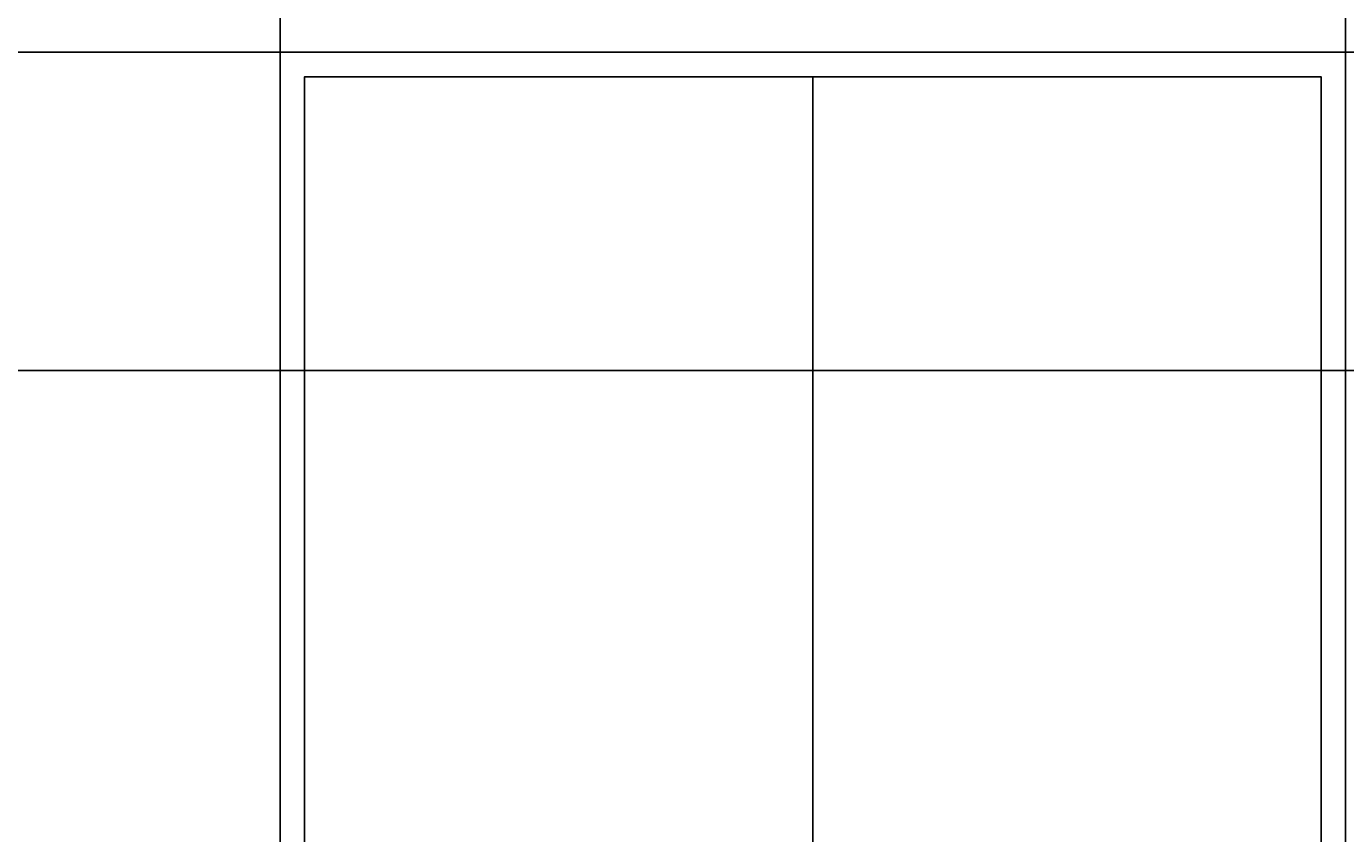
# Model space of a CAD drawing. Units: inches. Extents: x -145 to 510, y 5 to 386.
# Tile 12 of 25: x 75 to 182, y 242 to 308. Entities that reach past the tile are written whole.
import ezdxf

# ---------------------------------------------------------------- set-up
doc = ezdxf.new("R2010")
doc.units = ezdxf.units.IN
doc.header["$MEASUREMENT"] = 0
doc.layers.add('A-ANNO-DIMS', color=2, linetype='Continuous', lineweight=18)
doc.layers.add('A-GLAZ', color=4, linetype='Continuous', lineweight=25)
doc.styles.get("Standard").update_dxf_attribs({"font": 'arial.ttf'})
doc.dimstyles.get("Standard").update_dxf_attribs({"dimtxt": 0.6875, "dimasz": 0.18, "dimexe": 0.18, "dimexo": 0.0625, "dimgap": 0.09, "dimtad": 0, "dimtih": 1, "dimtoh": 1, "dimdec": 4, "dimzin": 0, "dimdsep": 46, "dimlunit": 4, "dimtxsty": 'Standard', "dimcen": 0.09, "dimadec": 0, "dimazin": 0, "dimtfac": 1, "dimtdec": 4, "dimtofl": 0, "dimtmove": 0, "dimatfit": 3, "dimfxl": 1, "dimtolj": 1, "dimtzin": 0, "dimarcsym": 0})

# ---------------------------------------------------------------- blocks, each defined once
blk = doc.blocks.new('*D15')
at = {"layer": 'A-ANNO-DIMS', "color": 0, "lineweight": -2, "transparency": 16777216}
for p, q in [((69.78, 199.95), (69.78, 385.97)), ((69.96, 385.79), (80.93, 385.79)), ((94.96, 385.79), (83.98, 385.79)), ((95.14, 305.8), (95.14, 385.97))]:
    blk.add_line(p, q, dxfattribs=at)
at = {"layer": 'A-ANNO-DIMS', "color": 0, "transparency": 16777216}
for points in [[(69.96, 385.82), (69.96, 385.76), (69.78, 385.79)], [(94.96, 385.82), (94.96, 385.76), (95.14, 385.79)]]:
    blk.add_solid(points, dxfattribs=at)
at = {"layer": 'Defpoints', "color": 0, "transparency": 16777216}
for p in [(95.14, 385.79), (95.14, 305.74), (69.78, 199.89)]:
    blk.add_point(p, dxfattribs=at)
at = {"layer": 'A-ANNO-DIMS', "color": 0, "transparency": 16777216, "insert": (82.46, 385.79), "char_height": 0.688, "attachment_point": 5}
blk.add_mtext('\\A1;25.365', dxfattribs=at)
blk = doc.blocks.new('*D16')
at = {"layer": 'A-ANNO-DIMS', "color": 0, "lineweight": -2, "transparency": 16777216}
for p, q in [((95.14, 305.8), (95.14, 385.97)), ((95.32, 385.79), (137.23, 385.79)), ((181.64, 385.79), (139.73, 385.79)), ((181.82, 305.8), (181.82, 385.97))]:
    blk.add_line(p, q, dxfattribs=at)
at = {"layer": 'A-ANNO-DIMS', "color": 0, "transparency": 16777216}
for points in [[(95.32, 385.82), (95.32, 385.76), (95.14, 385.79)], [(181.64, 385.82), (181.64, 385.76), (181.82, 385.79)]]:
    blk.add_solid(points, dxfattribs=at)
at = {"layer": 'Defpoints', "color": 0, "transparency": 16777216}
for p in [(181.82, 385.79), (95.14, 305.74), (181.82, 305.74)]:
    blk.add_point(p, dxfattribs=at)
at = {"layer": 'A-ANNO-DIMS', "color": 0, "transparency": 16777216, "insert": (138.48, 385.79), "char_height": 0.688, "attachment_point": 5}
blk.add_mtext('\\A1;86.68', dxfattribs=at)
blk = doc.blocks.new('*D19')
at = {"layer": 'A-ANNO-DIMS', "color": 0, "lineweight": -2, "transparency": 16777216}
for p, q in [((478.76, 355.89), (-144.05, 355.89)), ((-143.87, 355.71), (-143.87, 218.33)), ((-143.87, 80.07), (-143.87, 217.45)), ((-114.04, 79.89), (-144.05, 79.89))]:
    blk.add_line(p, q, dxfattribs=at)
at = {"layer": 'A-ANNO-DIMS', "color": 0, "transparency": 16777216}
for points in [[(-143.9, 355.71), (-143.84, 355.71), (-143.87, 355.89)], [(-143.9, 80.07), (-143.84, 80.07), (-143.87, 79.89)]]:
    blk.add_solid(points, dxfattribs=at)
at = {"layer": 'Defpoints', "color": 0, "transparency": 16777216}
for p in [(-143.87, 355.89), (478.83, 355.89), (-113.97, 79.89)]:
    blk.add_point(p, dxfattribs=at)
at = {"layer": 'A-ANNO-DIMS', "color": 0, "transparency": 16777216, "insert": (-143.87, 217.89), "char_height": 0.688, "attachment_point": 5}
blk.add_mtext('\\A1;276', dxfattribs=at)
blk = doc.blocks.new('*D26')
at = {"layer": 'A-ANNO-DIMS', "color": 0, "lineweight": -2, "transparency": 16777216}
for p, q in [((95.08, 305.74), (-144.05, 305.74)), ((-143.87, 305.56), (-143.87, 253.26)), ((-143.87, 200.07), (-143.87, 252.38)), ((95.08, 199.89), (-144.05, 199.89))]:
    blk.add_line(p, q, dxfattribs=at)
at = {"layer": 'A-ANNO-DIMS', "color": 0, "transparency": 16777216}
for points in [[(-143.9, 305.56), (-143.84, 305.56), (-143.87, 305.74)], [(-143.9, 200.07), (-143.84, 200.07), (-143.87, 199.89)]]:
    blk.add_solid(points, dxfattribs=at)
at = {"layer": 'Defpoints', "color": 0, "transparency": 16777216}
for p in [(-143.87, 305.74), (95.14, 305.74), (95.14, 199.89)]:
    blk.add_point(p, dxfattribs=at)
at = {"layer": 'A-ANNO-DIMS', "color": 0, "transparency": 16777216, "insert": (-143.87, 252.82), "char_height": 0.688, "attachment_point": 5}
blk.add_mtext('\\A1;105.85', dxfattribs=at)
blk = doc.blocks.new('*D27')
at = {"layer": 'A-ANNO-DIMS', "color": 0, "lineweight": -2, "transparency": 16777216}
for p, q in [((244.23, 279.84), (-144.05, 279.84)), ((-143.87, 279.66), (-143.87, 240.31)), ((-143.87, 200.07), (-143.87, 239.43)), ((218.29, 199.89), (-144.05, 199.89))]:
    blk.add_line(p, q, dxfattribs=at)
at = {"layer": 'A-ANNO-DIMS', "color": 0, "transparency": 16777216}
for points in [[(-143.9, 279.66), (-143.84, 279.66), (-143.87, 279.84)], [(-143.9, 200.07), (-143.84, 200.07), (-143.87, 199.89)]]:
    blk.add_solid(points, dxfattribs=at)
at = {"layer": 'Defpoints', "color": 0, "transparency": 16777216}
for p in [(-143.87, 279.84), (244.29, 279.84), (218.36, 199.89)]:
    blk.add_point(p, dxfattribs=at)
at = {"layer": 'A-ANNO-DIMS', "color": 0, "transparency": 16777216, "insert": (-143.87, 239.87), "char_height": 0.688, "attachment_point": 5}
blk.add_mtext('\\A1;79.95', dxfattribs=at)
blk = doc.blocks.new('*D28')
at = {"layer": 'A-ANNO-DIMS', "color": 0, "lineweight": -2, "transparency": 16777216}
for p, q in [((244.23, 305.74), (-144.05, 305.74)), ((-143.87, 305.56), (-143.87, 293.23)), ((-143.87, 280.02), (-143.87, 292.35)), ((244.23, 279.84), (-144.05, 279.84))]:
    blk.add_line(p, q, dxfattribs=at)
at = {"layer": 'A-ANNO-DIMS', "color": 0, "transparency": 16777216}
for points in [[(-143.9, 305.56), (-143.84, 305.56), (-143.87, 305.74)], [(-143.9, 280.02), (-143.84, 280.02), (-143.87, 279.84)]]:
    blk.add_solid(points, dxfattribs=at)
at = {"layer": 'Defpoints', "color": 0, "transparency": 16777216}
for p in [(-143.87, 305.74), (244.29, 305.74), (244.29, 279.84)]:
    blk.add_point(p, dxfattribs=at)
at = {"layer": 'A-ANNO-DIMS', "color": 0, "transparency": 16777216, "insert": (-143.87, 292.79), "char_height": 0.688, "attachment_point": 5}
blk.add_mtext('\\A1;25.897', dxfattribs=at)

msp = doc.modelspace()

# ---------------------------------------------------------------- linework, layer by layer
at = {"layer": 'A-GLAZ'}
msp.add_line((138.4805, 303.7416), (138.4805, 201.8905), dxfattribs=at)
for points in [[(95.1414, 199.8905), (181.8195, 199.8905), (181.8195, 305.7416), (95.1414, 305.7416)], [(97.1414, 201.8905), (179.8195, 201.8905), (179.8195, 303.7416), (97.1414, 303.7416)]]:
    msp.add_lwpolyline(points, close=True, dxfattribs=at)

# ---------------------------------------------------------------- dimensions: what is measured, and where the dimension line sits
at = {"layer": 'A-ANNO-DIMS'}
for base, p1, p2, override, picture, middle in [((95.1414, 385.7905), (69.7763, 199.8905), (95.1414, 305.7416), {"dimdec": 3, "dimlfac": 1, "dimrnd": 0, "dimzin": 0, "dimdsep": 46, "dimlunit": 2}, '*D15', (82.4589, 385.7905)), ((181.8195, 385.7905), (95.1414, 305.7416), (181.8195, 305.7416), {"dimdec": 2, "dimlfac": 1, "dimrnd": 0, "dimzin": 0, "dimdsep": 46, "dimlunit": 2}, '*D16', (138.4805, 385.7905))]:
    dim = msp.add_linear_dim(base=base, p1=p1, p2=p2, dimstyle='Standard', override=override, dxfattribs=at)
    dim.commit()
    dim.dimension.update_dxf_attribs({"geometry": picture, "text_midpoint": middle})
for base, p1, p2, override, picture, middle in [((-143.8737, 355.8905), (-113.9737, 79.8905), (478.8263, 355.8905), {"dimdec": 0, "dimlfac": 1, "dimrnd": 0, "dimzin": 0, "dimdsep": 46, "dimlunit": 2}, '*D19', (-143.8737, 217.8905)), ((-143.8737, 305.7416), (95.1414, 199.8905), (95.1414, 305.7416), {"dimdec": 2, "dimlfac": 1, "dimrnd": 0, "dimzin": 0, "dimdsep": 46, "dimlunit": 2}, '*D26', (-143.8737, 252.8161)), ((-143.8737, 305.7416), (244.2916, 279.8443), (244.2916, 305.7416), {"dimdec": 3, "dimlfac": 1, "dimrnd": 0, "dimzin": 0, "dimdsep": 46, "dimlunit": 2}, '*D28', (-143.8737, 292.793)), ((-143.8737, 279.8443), (218.3571, 199.8905), (244.2916, 279.8443), {"dimdec": 2, "dimlfac": 1, "dimrnd": 0, "dimzin": 0, "dimdsep": 46, "dimlunit": 2}, '*D27', (-143.8737, 239.8674))]:
    dim = msp.add_linear_dim(base=base, p1=p1, p2=p2, angle=90, dimstyle='Standard', override=override, dxfattribs=at)
    dim.commit()
    dim.dimension.update_dxf_attribs({"geometry": picture, "text_midpoint": middle})

doc.saveas('drawing.dxf')
